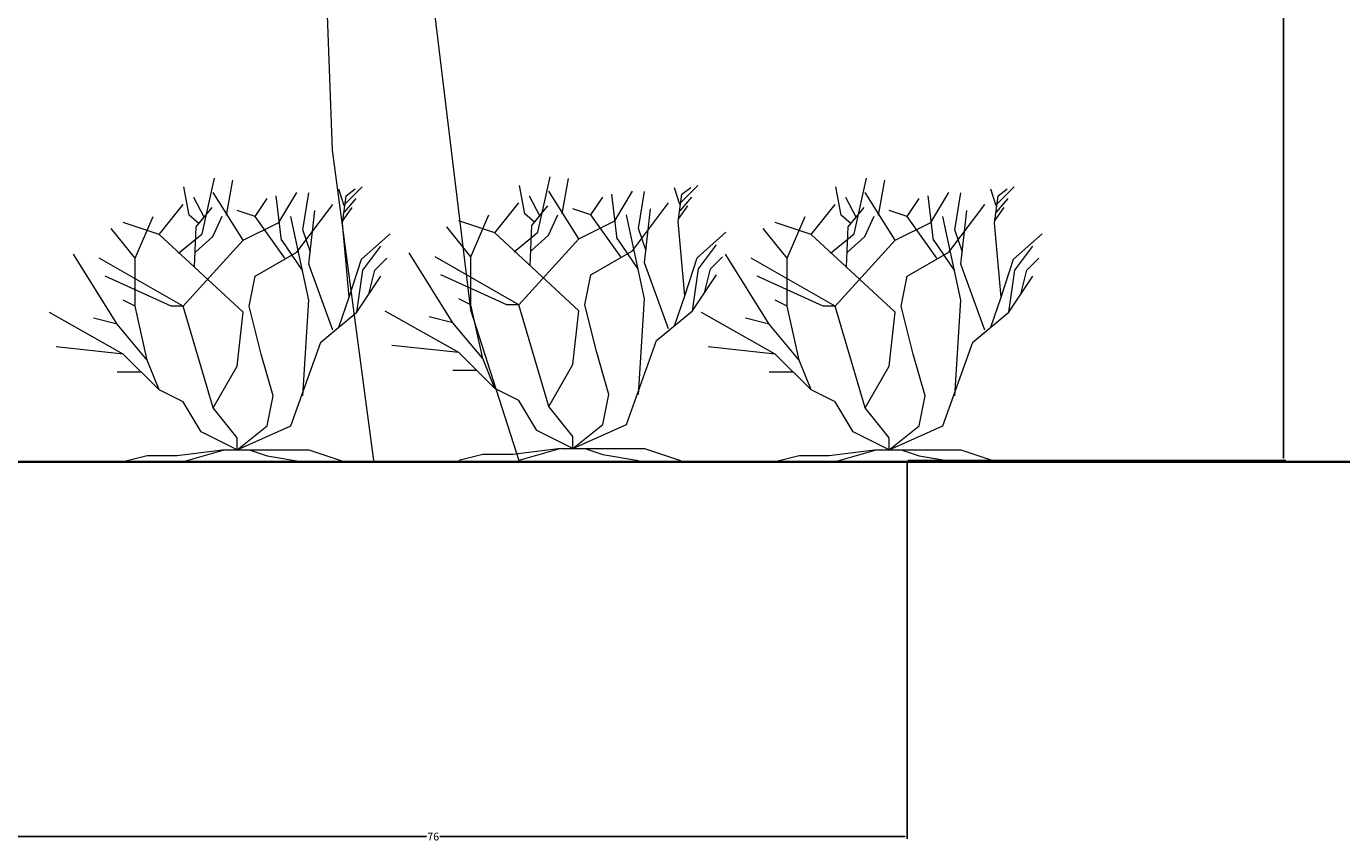
# Model space of a CAD drawing. Units: inches. Extents: x -13 to 809, y 112 to 656.
# Tile 43 of 55: x 641 to 747, y 120 to 185. Entities that reach past the tile are written whole.
import ezdxf

# ---------------------------------------------------------------- set-up
doc = ezdxf.new("R2010")
doc.units = ezdxf.units.IN
doc.header["$MEASUREMENT"] = 0
for name, color, linetype, lineweight in [('A-ANNO-DIMS', 2, 'Continuous', 18), ('A-ELEV', 7, 'Continuous', 35), ('L-PLNT', 3, 'Continuous', 18)]:
    doc.layers.add(name, color=color, linetype=linetype, lineweight=lineweight)
doc.styles.get("Standard").update_dxf_attribs({"font": 'arial.ttf'})
doc.dimstyles.get("Standard").update_dxf_attribs({"dimtxt": 0.625, "dimasz": 0.18, "dimexe": 0.18, "dimexo": 0.0625, "dimgap": 0.09, "dimtad": 0, "dimtih": 1, "dimtoh": 1, "dimdec": 4, "dimzin": 0, "dimdsep": 46, "dimlunit": 4, "dimtxsty": 'Standard', "dimcen": 0.09, "dimadec": 0, "dimazin": 0, "dimtfac": 1, "dimtdec": 4, "dimtofl": 0, "dimtmove": 0, "dimatfit": 3, "dimfxl": 1, "dimtolj": 1, "dimtzin": 0, "dimarcsym": 0})

# ---------------------------------------------------------------- blocks, each defined once
blk = doc.blocks.new('Tree - palm elevation')
for points in [[(-2.363, 170.553), (-3.88, 148.505), (-4.988, 69.634), (-3.325, 24.869), (0, 0)], [(-0.116, 162.848), (0.554, 143.532), (2.217, 96.635), (3.88, 44.054), (7.76, 12.079), (11.64, 0)]]:
    blk.add_lwpolyline(points)
blk = doc.blocks.new('Shrub - elevation')
for p, q in [((-11.433, 18.289), (-10.457, 22.749)), ((-9.48, 19.775), (-8.992, 22.592)), ((-12.471, 19.775), (-12.898, 22.044)), ((-11.28, 19.619), (-12.104, 21.184)), ((-8.16, 17.76), (-10.56, 21.6)), ((-7.2, 19.68), (-6.24, 21.12)), ((-5.086, 17.741), (-5.513, 21.34)), ((-5.28, 19.2), (-3.84, 21.6)), ((-3.377, 18.602), (-2.888, 21.575)), ((-0.508, 21.888), (-0.081, 20.558)), ((-0.203, 19.149), (0.102, 21.34)), ((-0.02, 20.01), (0.896, 21.105)), ((0.041, 20.714), (1.384, 22.044)), ((0.102, 21.34), (0.835, 21.888)), ((-14.88, 18.24), (-12.96, 20.64)), ((-11.921, 18.836), (-10.64, 20.401)), ((-7.2, 19.68), (-8.64, 20.16)), ((-3.84, 16.8), (-0.96, 20.64)), ((-2.88, 15.84), (-2.4, 20.16)), ((-0.142, 19.384), (0.59, 20.401)), ((-14.88, 18.24), (-17.76, 19.2)), ((-16.8, 16.32), (-15.36, 19.68)), ((-11.677, 19.071), (-12.471, 19.775)), ((-10.579, 18.054), (-9.846, 19.697)), ((-8.16, 17.76), (-5.28, 19.2)), ((-4.8, 16.32), (-7.2, 19.68)), ((-2.88, 12.96), (-4.32, 19.68)), ((0.346, 13.203), (-0.203, 19.149)), ((-16.8, 16.32), (-18.72, 18.72)), ((-8.16, 12), (-14.88, 18.24)), ((-13.325, 16.724), (-11.433, 18.289)), ((-12.043, 15.628), (-11.921, 18.836)), ((-11.982, 16.802), (-10.579, 18.054)), ((-2.766, 16.802), (-3.377, 18.602)), ((1.323, 16.254), (3.642, 18.289)), ((-12.96, 12.48), (-8.16, 17.76)), ((-3.377, 15.315), (-5.086, 17.819)), ((1.44, 15.36), (2.88, 17.28)), ((-18.24, 11.04), (-21.755, 16.655)), ((-12.96, 12.48), (-19.68, 16.32)), ((-16.8, 12.48), (-16.8, 16.32)), ((-7.2, 14.88), (-3.84, 16.8)), ((-0.96, 10.56), (-2.88, 15.84)), ((0.346, 13.203), (1.323, 16.254)), ((2.4, 15.36), (3.36, 16.32)), ((-13.92, 12.48), (-19.2, 14.88)), ((-7.68, 12.48), (-7.2, 14.88)), ((0.96, 12), (1.44, 15.36)), ((0.96, 12), (2.88, 14.88)), ((1.92, 13.44), (2.4, 15.36)), ((-16.8, 12.48), (-17.76, 12.96)), ((-3.36, 5.28), (-2.88, 12.96)), ((-0.48, 10.8), (0.346, 13.203)), ((-17.76, 8.64), (-23.663, 11.961)), ((-15.84, 8.16), (-16.8, 12.48)), ((-12.96, 12.48), (-13.92, 12.48)), ((-10.56, 4.32), (-12.96, 12.48)), ((-8.64, 7.68), (-8.16, 12)), ((-6.72, 8.64), (-7.68, 12.48)), ((-1.92, 9.6), (0.96, 12)), ((-18.24, 11.04), (-20.16, 11.52)), ((-15.84, 8.16), (-18.24, 11.04)), ((-4.32, 2.88), (-1.92, 9.6)), ((-17.76, 8.64), (-23.128, 9.222)), ((-14.88, 5.76), (-17.76, 8.64)), ((-5.76, 5.28), (-6.72, 8.64)), ((-14.88, 5.76), (-15.84, 8.16)), ((-10.56, 4.32), (-8.64, 7.68)), ((-16.32, 7.2), (-18.24, 7.2)), ((-12.96, 4.8), (-14.88, 5.76)), ((-6.24, 2.88), (-5.76, 5.28)), ((-11.52, 2.4), (-12.96, 4.8)), ((-8.64, 1.92), (-10.56, 4.32)), ((-8.64, 0.96), (-11.52, 2.4)), ((-8.64, 0.96), (-4.32, 2.88)), ((-8.64, 0.96), (-6.24, 2.88)), ((-8.64, 0.96), (-8.64, 1.92)), ((-15.84, 0.48), (-17.76, 0)), ((-13.44, 0.48), (-15.84, 0.48)), ((-9.6, 0.96), (-13.44, 0.48)), ((-9.6, 0.96), (-12.96, 0)), ((-9.6, 0.96), (-7.68, 0.96)), ((-8.64, 0.96), (-2.88, 0.96)), ((-7.68, 0.96), (-6.24, 0.48)), ((-6.24, 0.48), (-3.36, 0)), ((-2.88, 0.96), (0, 0))]:
    blk.add_line(p, q)
blk = doc.blocks.new('*D9')
at = {"layer": 'A-ANNO-DIMS', "color": 0, "lineweight": -2, "transparency": 16777216}
for p, q in [((711.81, 351.8), (742.1, 351.8)), ((741.92, 351.62), (741.92, 251.63)), ((741.92, 150.81), (741.92, 250.81)), ((711.81, 150.63), (742.1, 150.63))]:
    blk.add_line(p, q, dxfattribs=at)
at = {"layer": 'A-ANNO-DIMS', "color": 0, "transparency": 16777216}
for points in [[(741.89, 351.62), (741.95, 351.62), (741.92, 351.8)], [(741.89, 150.81), (741.95, 150.81), (741.92, 150.63)]]:
    blk.add_solid(points, dxfattribs=at)
at = {"layer": 'Defpoints', "color": 0, "transparency": 16777216}
for p in [(711.75, 351.8), (741.92, 351.8), (711.75, 150.63)]:
    blk.add_point(p, dxfattribs=at)
at = {"layer": 'A-ANNO-DIMS', "color": 0, "transparency": 16777216, "insert": (741.92, 251.22), "char_height": 0.625, "attachment_point": 5}
blk.add_mtext('\\A1;PALM TREE 201', dxfattribs=at)
blk = doc.blocks.new('*D10')
at = {"layer": 'A-ANNO-DIMS', "color": 0, "lineweight": -2, "transparency": 16777216}
for p, q in [((635.78, 150.57), (635.78, 120.28)), ((711.75, 150.57), (711.75, 120.28)), ((635.96, 120.46), (673.23, 120.46)), ((711.57, 120.46), (674.3, 120.46))]:
    blk.add_line(p, q, dxfattribs=at)
at = {"layer": 'A-ANNO-DIMS', "color": 0, "transparency": 16777216}
for points in [[(635.96, 120.49), (635.96, 120.43), (635.78, 120.46)], [(711.57, 120.49), (711.57, 120.43), (711.75, 120.46)]]:
    blk.add_solid(points, dxfattribs=at)
at = {"layer": 'Defpoints', "color": 0, "transparency": 16777216}
for p in [(635.78, 150.63), (711.75, 150.63), (711.75, 120.46)]:
    blk.add_point(p, dxfattribs=at)
at = {"layer": 'A-ANNO-DIMS', "color": 0, "transparency": 16777216, "insert": (673.77, 120.46), "char_height": 0.625, "attachment_point": 5}
blk.add_mtext('\\A1;76', dxfattribs=at)
blk = doc.blocks.new('*D31')
at = {"layer": 'A-ANNO-DIMS', "color": 0, "lineweight": -2, "transparency": 16777216}
for p, q in [((621.07, 617.78), (807.77, 617.78)), ((807.59, 617.6), (807.59, 384.56)), ((807.59, 150.7), (807.59, 383.74)), ((621.07, 150.52), (807.77, 150.52))]:
    blk.add_line(p, q, dxfattribs=at)
at = {"layer": 'A-ANNO-DIMS', "color": 0, "transparency": 16777216}
for points in [[(807.56, 617.6), (807.62, 617.6), (807.59, 617.78)], [(807.56, 150.7), (807.62, 150.7), (807.59, 150.52)]]:
    blk.add_solid(points, dxfattribs=at)
at = {"layer": 'Defpoints', "color": 0, "transparency": 16777216}
for p in [(621.01, 617.78), (807.59, 617.78), (621.01, 150.52)]:
    blk.add_point(p, dxfattribs=at)
at = {"layer": 'A-ANNO-DIMS', "color": 0, "transparency": 16777216, "insert": (807.59, 384.15), "char_height": 0.625, "attachment_point": 5}
blk.add_mtext('\\A1;467.3', dxfattribs=at)
blk = doc.blocks.new('*D129')
at = {"layer": 'A-ANNO-DIMS', "color": 0, "lineweight": -2, "transparency": 16777216}
for p, q in [((607.64, 209.88), (807.77, 209.88)), ((807.59, 209.7), (807.59, 180.61)), ((807.59, 150.7), (807.59, 179.79)), ((608.76, 150.52), (807.77, 150.52))]:
    blk.add_line(p, q, dxfattribs=at)
at = {"layer": 'A-ANNO-DIMS', "color": 0, "transparency": 16777216}
for points in [[(807.56, 209.7), (807.62, 209.7), (807.59, 209.88)], [(807.56, 150.7), (807.62, 150.7), (807.59, 150.52)]]:
    blk.add_solid(points, dxfattribs=at)
at = {"layer": 'Defpoints', "color": 0, "transparency": 16777216}
for p in [(607.57, 209.88), (807.59, 209.88), (608.69, 150.52)]:
    blk.add_point(p, dxfattribs=at)
at = {"layer": 'A-ANNO-DIMS', "color": 0, "transparency": 16777216, "insert": (807.59, 180.2), "char_height": 0.625, "attachment_point": 5}
blk.add_mtext('\\A1;59.36', dxfattribs=at)

msp = doc.modelspace()

# ---------------------------------------------------------------- linework, layer by layer
at = {"layer": 'A-ELEV'}
for p, q in [((109.5888, 150.5199), (649.5888, 150.5199)), ((649.5888, 150.5199), (769.5888, 150.5199))]:
    msp.add_line(p, q, dxfattribs=at)

# ---------------------------------------------------------------- block references
at = {"layer": 'L-PLNT'}
for name, p in [('Tree - palm elevation', (668.9925, 150.6343)), ('Shrub - elevation', (666.6887, 150.5199)), ('Shrub - elevation', (693.5925, 150.6343)), ('Shrub - elevation', (718.9442, 150.5199))]:
    msp.add_blockref(name, p, dxfattribs=at)

# ---------------------------------------------------------------- dimensions: what is measured, and where the dimension line sits
at = {"layer": 'A-ANNO-DIMS'}
for base, p1, p2, override, picture, middle in [((807.5888, 617.7828), (621.008, 150.5199), (621.008, 617.7828), {"dimdec": 1, "dimlfac": 1, "dimrnd": 0, "dimzin": 0, "dimdsep": 46, "dimlunit": 2}, '*D31', (807.5888, 384.1514)), ((807.5888, 209.8753), (608.694, 150.5199), (607.5741, 209.8753), {"dimdec": 2, "dimlfac": 1, "dimrnd": 0, "dimzin": 0, "dimdsep": 46, "dimlunit": 2}, '*D129', (807.5888, 180.1976))]:
    dim = msp.add_linear_dim(base=base, p1=p1, p2=p2, angle=90, dimstyle='Standard', override=override, dxfattribs=at)
    dim.commit()
    dim.dimension.update_dxf_attribs({"geometry": picture, "text_midpoint": middle})
dim = msp.add_linear_dim(base=(741.9246, 351.8013), p1=(711.7495, 150.6343), p2=(711.7495, 351.8013), angle=90, text='PALM TREE <>', dimstyle='Standard', override={"dimdec": 0, "dimlfac": 1, "dimrnd": 0, "dimzin": 0, "dimdsep": 46, "dimlunit": 2}, dxfattribs=at)
dim.commit()
dim.dimension.update_dxf_attribs({"geometry": '*D9', "text_midpoint": (741.9246, 251.2178)})
dim = msp.add_linear_dim(base=(711.7495, 120.4592), p1=(635.7844, 150.6343), p2=(711.7495, 150.6343), dimstyle='Standard', override={"dimdec": 0, "dimlfac": 1, "dimrnd": 0, "dimzin": 0, "dimdsep": 46, "dimlunit": 2}, dxfattribs=at)
dim.commit()
dim.dimension.update_dxf_attribs({"geometry": '*D10', "text_midpoint": (673.7669, 120.4592)})

doc.saveas('drawing.dxf')
